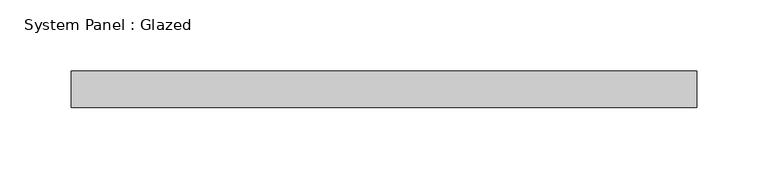
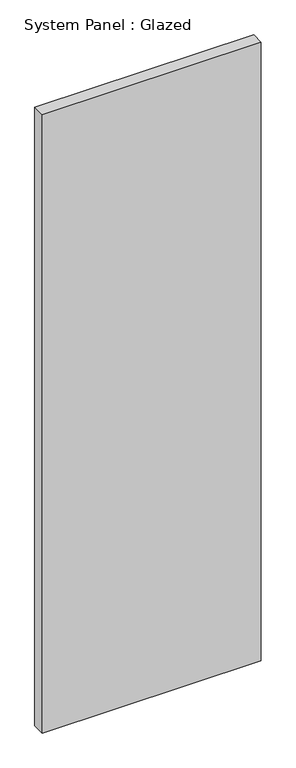
"""IFC4 building model written with IfcOpenShell, lengths in millimetres: plate geometry, System Panel : Glazed."""

from ifc_helpers import new_model, si_unit, origin, origin_with_axes, place, context, project, spatial, polyline, outline, extrude, source, transform, mapped, element, save


def system_panel_glazed_1572ce70(model_context):
    return source(origin(), model_context, "Body", "SweptSolid", [
        extrude(outline(polyline([(219.075, 19.05), (-219.075, 19.05), (-219.075, 44.45), (219.075, 44.45), (219.075, 19.05)])), origin_with_axes(), (0.0, 0.0, 1.0), 1306.7701004),
    ])


if __name__ == "__main__":
    model = new_model("IFC4")
    model_context = context("Model", 3, world=origin())
    ifc_project = project(units=[si_unit("LENGTHUNIT", "METRE", prefix="MILLI")], contexts=[model_context])
    site = spatial("IfcSite", under=ifc_project)
    building = spatial("IfcBuilding", under=site)
    placement = place(None, origin())
    system_panel_glazed_shape = system_panel_glazed_1572ce70(model_context)
    element("IfcPlate", 1, ObjectType="System Panel : Glazed", at=placement, inside=building, context=model_context, shape_type="MappedRepresentation", body=[
        mapped(system_panel_glazed_shape, transform((0.0, 0.0, 0.0), x_axis=(1.0, 0.0, 0.0), y_axis=(0.0, 1.0, 0.0), z_axis=(0.0, 0.0, 1.0))),
    ])
    save(model, "model.ifc")

# Revit data of these elements
# Type "System Panel : Glazed"
#   Construction Type Id = "GSP4R"
#   Analytic Construction = "1/8 in Pilkington single glazing"
#   Visual Light Transmittance = 0.9
#   Solar Heat Gain Coefficient = 0.86
#   Heat Transfer Coefficient (U) = 1.18115 BTU/(h·ft²·°F)
#   Define Thermal Properties by = 1
# Element 1 (IfcPlate, "System Panel : Glazed")
#   Materials on its faces: "Glass"
# Materials
#   "Glass": class "Glass", colour RGB 0 128 192, transparency 0.75, Description = "Soda Lime Glass", Cost = 0
